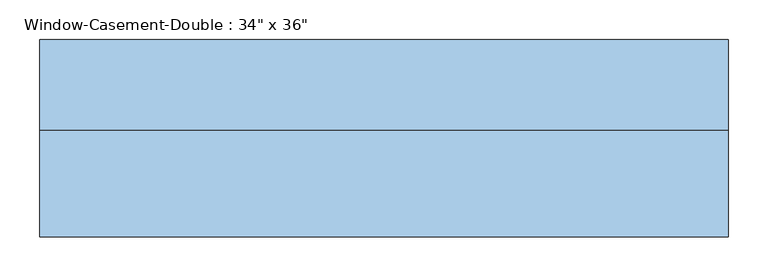
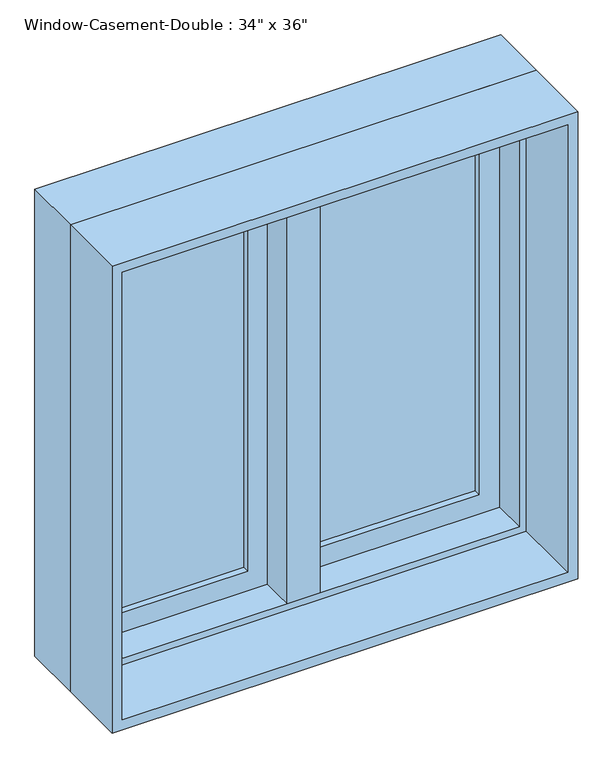
"""IFC4 building model written with IfcOpenShell, lengths in millimetres: window geometry."""

from ifc_helpers import new_model, si_unit, frame, origin, place, context, project, spatial, polyline, outline, extrude, faceted_brep, source, transform, mapped, element, save


def window_339605e1(model_context):
    return source(origin(), model_context, "Body", "SolidModel", [
        faceted_brep([(9.525, 133.35, 1816.1), (-9.525, 133.35, 1816.1), (-9.525, 82.55, 1816.1), (9.525, 82.55, 1816.1), (9.525, 133.35, 927.1), (9.525, 82.55, 927.1), (-9.525, 82.55, 927.1), (-9.525, 133.35, 927.1), (-9.525, 82.55, 946.15), (-9.525, 82.55, 1797.05), (-30.1625, 82.55, 946.15), (-30.1625, 82.55, 1797.05), (-30.1625, 19.05, 946.15), (-30.1625, 19.05, 1797.05), (30.1625, 19.05, 946.15), (30.1625, 19.05, 1797.05), (30.1625, 82.55, 946.15), (30.1625, 82.55, 1797.05), (9.525, 82.55, 946.15), (9.525, 82.55, 1797.05)], [[[0, 1, 2, 3]], [[4, 5, 6, 7]], [[1, 0, 4, 7]], [[2, 1, 7, 6, 8, 9]], [[9, 8, 10, 11]], [[11, 10, 12, 13]], [[13, 12, 14, 15]], [[15, 14, 16, 17]], [[17, 16, 18, 19]], [[0, 3, 19, 18, 5, 4]], [[18, 8, 6, 5]], [[9, 19, 3, 2]], [[8, 18, 16, 14, 12, 10]], [[19, 9, 11, 13, 15, 17]]]),
        extrude(outline(polyline([(-66.675, 114.3), (-66.675, 107.95), (-361.95, 107.95), (-361.95, 114.3), (-66.675, 114.3)])), frame((0.0, 0.0, 984.25), z_axis=(0.0, 0.0, 1.0), x_axis=(1.0, 0.0, 0.0)), (0.0, 0.0, 1.0), 774.7),
        extrude(outline(polyline([(-361.95, 95.25), (-361.95, 101.6), (-66.675, 101.6), (-66.675, 95.25), (-361.95, 95.25)])), frame((0.0, 0.0, 984.25), z_axis=(0.0, 0.0, 1.0), x_axis=(1.0, 0.0, 0.0)), (0.0, 0.0, 1.0), 774.7),
        extrude(outline(polyline([(361.95, 114.3), (361.95, 107.95), (66.675, 107.95), (66.675, 114.3), (361.95, 114.3)])), frame((0.0, 0.0, 984.25), z_axis=(0.0, 0.0, 1.0), x_axis=(1.0, 0.0, 0.0)), (0.0, 0.0, 1.0), 774.7),
        extrude(outline(polyline([(66.675, 95.25), (66.675, 101.6), (361.95, 101.6), (361.95, 95.25), (66.675, 95.25)])), frame((0.0, 0.0, 984.25), z_axis=(0.0, 0.0, 1.0), x_axis=(1.0, 0.0, 0.0)), (0.0, 0.0, 1.0), 774.7),
        extrude(outline(polyline([(1816.1, -419.1), (927.1, -419.1), (927.1, -9.525), (1816.1, -9.525), (1816.1, -419.1)]), holes=[polyline([(1758.95, -66.675), (984.25, -66.675), (984.25, -361.95), (1758.95, -361.95), (1758.95, -66.675)])]), frame((0.0, 82.55, 0.0), z_axis=(0.0, 1.0, 0.0), x_axis=(0.0, 0.0, 1.0)), (0.0, 0.0, 1.0), 44.45),
        extrude(outline(polyline([(927.1, 419.1), (1816.1, 419.1), (1816.1, 9.525), (927.1, 9.525), (927.1, 419.1)]), holes=[polyline([(984.25, 66.675), (1758.95, 66.675), (1758.95, 361.95), (984.25, 361.95), (984.25, 66.675)])]), frame((0.0, 82.55, 0.0), z_axis=(0.0, 1.0, 0.0), x_axis=(0.0, 0.0, 1.0)), (0.0, 0.0, 1.0), 44.45),
        extrude(outline(polyline([(1828.8, -431.8), (914.4, -431.8), (914.4, 431.8), (1828.8, 431.8), (1828.8, -431.8)]), holes=[polyline([(1809.75, 412.75), (933.45, 412.75), (933.45, -412.75), (1809.75, -412.75), (1809.75, 412.75)])]), frame((0.0, -114.3, 0.0), z_axis=(0.0, 1.0, 0.0), x_axis=(0.0, 0.0, 1.0)), (0.0, 0.0, 1.0), 133.35),
        faceted_brep([(400.05, 82.55, 1797.05), (400.05, 19.05, 1797.05), (-400.05, 19.05, 1797.05), (-400.05, 82.55, 1797.05), (419.1, 133.35, 1816.1), (419.1, 82.55, 1816.1), (-419.1, 82.55, 1816.1), (-419.1, 133.35, 1816.1), (431.8, 19.05, 1828.8), (431.8, 133.35, 1828.8), (-431.8, 133.35, 1828.8), (-431.8, 19.05, 1828.8), (-400.05, 19.05, 946.15), (-400.05, 82.55, 946.15), (-419.1, 82.55, 927.1), (-419.1, 133.35, 927.1), (-431.8, 133.35, 914.4), (-431.8, 19.05, 914.4), (400.05, 19.05, 946.15), (400.05, 82.55, 946.15), (419.1, 82.55, 927.1), (419.1, 133.35, 927.1), (431.8, 133.35, 914.4), (431.8, 19.05, 914.4)], [[[0, 1, 2, 3]], [[4, 5, 6, 7]], [[8, 9, 10, 11]], [[3, 2, 12, 13]], [[7, 6, 14, 15]], [[11, 10, 16, 17]], [[13, 12, 18, 19]], [[15, 14, 20, 21]], [[17, 16, 22, 23]], [[11, 17, 23, 8], [1, 18, 12, 2]], [[19, 18, 1, 0]], [[5, 20, 14, 6], [3, 13, 19, 0]], [[21, 20, 5, 4]], [[23, 22, 9, 8]], [[9, 22, 16, 10], [7, 15, 21, 4]]]),
    ])


if __name__ == "__main__":
    model = new_model("IFC4")
    model_context = context("Model", 3, world=origin())
    ifc_project = project(units=[si_unit("LENGTHUNIT", "METRE", prefix="MILLI")], contexts=[model_context])
    site = spatial("IfcSite", under=ifc_project)
    building = spatial("IfcBuilding", under=site)
    placement = place(None, origin())
    window_shape = window_339605e1(model_context)
    element("IfcWindow", 1, ObjectType="Window-Casement-Double : 34\" x 36\"", at=placement, inside=building, context=model_context, shape_type="MappedRepresentation", body=[
        mapped(window_shape, transform((0.0, 0.0, 0.0), x_axis=(1.0, 0.0, 0.0), y_axis=(0.0, 1.0, 0.0), z_axis=(0.0, 0.0, 1.0))),
    ])
    save(model, "model.ifc")

# Revit data of these elements
# Type "Window-Casement-Double : 34\" x 36\""
#   Type Mark = "14"
#   Fire Rating = "0.5h"
#   Assembly Code = "B2020100"
#   Analytic Construction = "Double glazing - domestic"
#   Frame Extension [instance default] = 0' - 0 1/4"
#   Window Inset [instance default] = 0' - 0"
#   Wall Thickness [instance default] = 0' - 6"
#   Interior Wall Closure [instance default] = 0' - 2 1/4"
#   Half Width = 1' - 5"
#   Visual Light Transmittance = 0.81
#   Thermal Resistance (R) = 1.8146 (h·ft²·°F)/BTU
#   Solar Heat Gain Coefficient = 0.76
#   Rough Width = 2' - 10 1/2"
#   Rough Height = 3' - 0 1/2"
#   Height = 3' - 0"
#   Heat Transfer Coefficient (U) = 0.5511 BTU/(h·ft²·°F)
#   Exterior Wall Closure [instance default] = 0' - 1 1/4"
#   Extension Jamb [instance default] = 0' - 2 1/4"
#   Default Sill Height = 3' - 0"
#   Width = 2' - 10"
#   Define Thermal Properties by = 0
#   Muntin Visibility = yes
#   Interior Trim Visibility [instance default] = yes
#   Exterior Trim Visibility [instance default] = yes
#   Extension Jamb Visibility [instance default] = yes
#   Interior Trim Material = Wood - Stained
#   Muntin Pattern = Muntin Pattern_2x2 : Muntin Pattern_2x2
#   Interior Trim = Trim-Window-Interior-Flat : Picture Frame
#   Interior Frame Material = Wood - Stained
#   Glass Panel Material = Glass
#   Exterior Trim Material = Clad - White
#   Exterior Trim = Trim-Window-Exterior-Flat : with Sill
#   Exterior Frame Material = Clad - White
#   Wall Closure = (empty or 0)
# Element 1 (IfcWindow, "Window-Casement-Double : 34\" x 36\"")
#   Wall Thickness = 0' - 9"
#   Extension Jamb = 0' - 5 1/4"
#   Materials on its faces: "Wood - Stained", "Glass", "Clad - White"
# Materials
#   "Wood - Stained": class "Wood", colour RGB 224 178 126, transparency 0, Cost = 0
#   "Glass": class "Glass", colour RGB 0 128 192, transparency 0.75, Description = "Soda Lime Glass", Cost = 0
#   "Clad - White": class "Wood", colour RGB 30 30 30, transparency 0, Cost = 0
